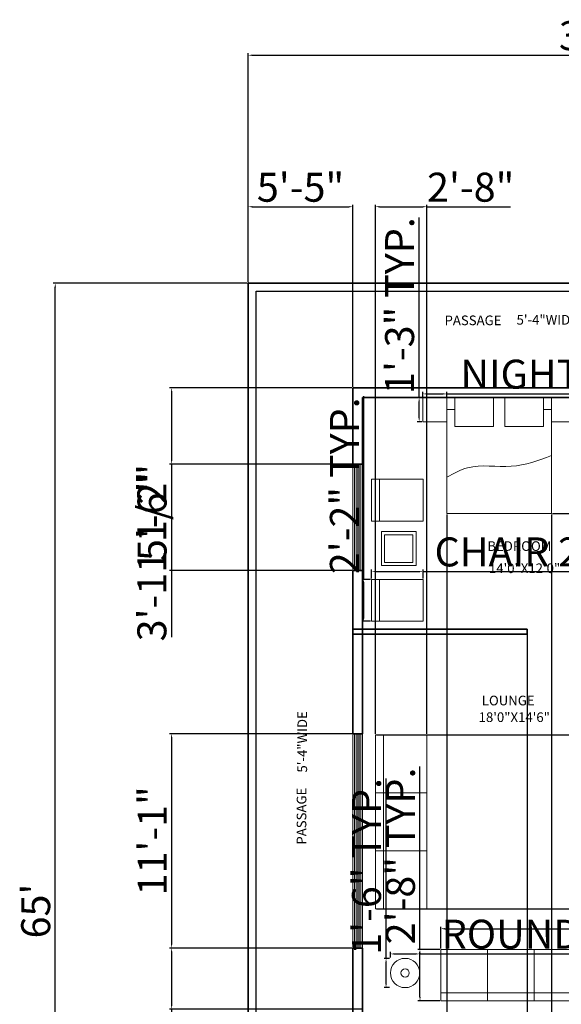
# Model space of a CAD drawing. Units: inches. Extents: x 2484 to 3244, y 1684 to 2692.
# Tile 2 of 3: x 2484 to 2821, y 2081 to 2692. Entities that reach past the tile are written whole.
import ezdxf

# ---------------------------------------------------------------- set-up
doc = ezdxf.new("R2010")
doc.units = ezdxf.units.IN
doc.layers.get('0').update_dxf_attribs({"color": 120})
for name, color, linetype, lineweight in [('A-ANNO-DIMS', 2, 'Continuous', 18), ('A-AREA-IDEN', 2, 'Continuous', 18), ('A-FURN', 40, 'Continuous', 18), ('A-GLAZ', 4, 'Continuous', 13), ('A-WALL', 120, 'Continuous', 35), ('C-PROP', 120, 'Continuous', 35), ('C-SITE', 120, 'Continuous', 25)]:
    doc.layers.add(name, color=color, linetype=linetype, lineweight=lineweight)
doc.styles.get("Standard").update_dxf_attribs({"font": 'arial.ttf'})
doc.dimstyles.new('ISO-25', dxfattribs={"dimtxt": 18, "dimasz": 2.5, "dimexe": 1.25, "dimexo": 0.625, "dimtad": 1, "dimdec": 0, "dimlunit": 3, "dimtxsty": 'Standard', "dimcen": 2.5, "dimadec": 0, "dimazin": 0, "dimtfac": 1, "dimtdec": 0, "dimtmove": 0, "dimatfit": 3, "dimfxl": 1, "dimarcsym": 0})

# ---------------------------------------------------------------- blocks, each defined once
blk = doc.blocks.new('*D1')
at = {"layer": 'A-ANNO-DIMS', "color": 0, "lineweight": -2, "transparency": 16777216}
for p, q in [((2626.09, 2529.34), (2626.09, 2671.64)), ((2628.59, 2670.39), (3043.59, 2670.39)), ((3046.09, 2529.34), (3046.09, 2671.64))]:
    blk.add_line(p, q, dxfattribs=at)
at = {"layer": 'A-ANNO-DIMS', "color": 0, "transparency": 16777216}
for points in [[(2628.59, 2670.81), (2628.59, 2669.97), (2626.09, 2670.39)], [(3043.59, 2670.81), (3043.59, 2669.97), (3046.09, 2670.39)]]:
    blk.add_solid(points, dxfattribs=at)
at = {"layer": 'Defpoints', "color": 0, "transparency": 16777216}
for p in [(3046.09, 2670.39), (2626.09, 2528.71), (3046.09, 2528.71)]:
    blk.add_point(p, dxfattribs=at)
at = {"layer": 'A-ANNO-DIMS', "color": 0, "transparency": 16777216, "insert": (2836.09, 2680.21), "char_height": 18, "attachment_point": 5}
blk.add_mtext("35'", dxfattribs=at)
blk = doc.blocks.new('*D2')
at = {"layer": 'A-ANNO-DIMS', "color": 0, "lineweight": -2, "transparency": 16777216}
for p, q in [((2625.46, 2528.71), (2505.02, 2528.71)), ((2506.27, 1751.21), (2506.27, 2526.21)), ((2625.46, 1748.71), (2505.02, 1748.71))]:
    blk.add_line(p, q, dxfattribs=at)
at = {"layer": 'A-ANNO-DIMS', "color": 0, "transparency": 16777216}
for points in [[(2505.85, 2526.21), (2506.68, 2526.21), (2506.27, 2528.71)], [(2505.85, 1751.21), (2506.68, 1751.21), (2506.27, 1748.71)]]:
    blk.add_solid(points, dxfattribs=at)
at = {"layer": 'Defpoints', "color": 0, "transparency": 16777216}
for p in [(2506.27, 2528.71), (2626.09, 2528.71), (2626.09, 1748.71)]:
    blk.add_point(p, dxfattribs=at)
at = {"layer": 'A-ANNO-DIMS', "color": 0, "transparency": 16777216, "insert": (2496.45, 2138.71), "char_height": 18, "attachment_point": 5, "rotation": 90}
blk.add_mtext("65'", dxfattribs=at)
blk = doc.blocks.new('SOFA-3')
for p, q in [((0.07, 0), (0.07, 32)), ((0.07, 32), (86.07, 32)), ((29.07, 0), (29.07, 32)), ((58.07, 0), (58.07, 32)), ((86.07, 32), (86.07, 0)), ((0.07, 0), (0, 5)), ((0, 5), (86.07, 5)), ((0.07, 0), (0.07, 5)), ((86.07, 0), (0.07, 0))]:
    blk.add_line(p, q)
blk = doc.blocks.new('CHAIR')
for p, q in [((0, 26), (5, 26)), ((5, 26), (5, 0))]:
    blk.add_line(p, q)
blk.add_lwpolyline([(0, 0), (32, 0), (32, 26), (0, 26)], close=True)
blk = doc.blocks.new('TABLE-ROUND')
for radius in [9.1, 2.6]:
    blk.add_circle((0, 0), radius)
blk = doc.blocks.new('NIGHTSTAND-15')
blk.add_lwpolyline([(15, 15), (0, 15), (0, 0), (15, 0)], close=True)
blk = doc.blocks.new('*D9')
at = {"layer": 'A-ANNO-DIMS', "color": 0, "lineweight": -2, "transparency": 16777216}
for p, q in [((2714.44, 2109.91), (2714.44, 2113.27)), ((2716.94, 2112.02), (2730.14, 2112.02)), ((2732.64, 2109.91), (2732.64, 2113.27)), ((2732.64, 2112.02), (3096.69, 2112.02))]:
    blk.add_line(p, q, dxfattribs=at)
at = {"layer": 'A-ANNO-DIMS', "color": 0, "transparency": 16777216}
for points in [[(2716.94, 2112.44), (2716.94, 2111.6), (2714.44, 2112.02)], [(2730.14, 2112.44), (2730.14, 2111.6), (2732.64, 2112.02)]]:
    blk.add_solid(points, dxfattribs=at)
at = {"layer": 'Defpoints', "color": 0, "transparency": 16777216}
for p in [(2732.64, 2112.02), (2714.44, 2109.29), (2732.64, 2109.29)]:
    blk.add_point(p, dxfattribs=at)
at = {"layer": 'A-ANNO-DIMS', "color": 0, "transparency": 16777216, "insert": (2915.92, 2121.96), "char_height": 18, "attachment_point": 5}
blk.add_mtext('ROUND SIDE TABLE 1\'-6" TYP.', dxfattribs=at)
blk = doc.blocks.new('*D10')
at = {"layer": 'A-ANNO-DIMS', "color": 0, "lineweight": -2, "transparency": 16777216}
for p, q in [((2711.71, 2109.29), (2711.71, 2221.06)), ((2713.81, 2109.29), (2710.46, 2109.29)), ((2711.71, 2093.58), (2711.71, 2106.79)), ((2713.81, 2091.08), (2710.46, 2091.08))]:
    blk.add_line(p, q, dxfattribs=at)
at = {"layer": 'A-ANNO-DIMS', "color": 0, "transparency": 16777216}
for points in [[(2711.29, 2106.79), (2712.12, 2106.79), (2711.71, 2109.29)], [(2711.29, 2093.58), (2712.12, 2093.58), (2711.71, 2091.08)]]:
    blk.add_solid(points, dxfattribs=at)
at = {"layer": 'Defpoints', "color": 0, "transparency": 16777216}
for p in [(2711.71, 2109.29), (2714.44, 2109.29), (2714.44, 2091.08)]:
    blk.add_point(p, dxfattribs=at)
at = {"layer": 'A-ANNO-DIMS', "color": 0, "transparency": 16777216, "insert": (2701.89, 2166.43), "char_height": 18, "attachment_point": 5, "rotation": 90}
blk.add_mtext('1\'-6" TYP.', dxfattribs=at)
blk = doc.blocks.new('*D13')
at = {"layer": 'A-ANNO-DIMS', "color": 0, "lineweight": -2, "transparency": 16777216}
for p, q in [((2745.68, 2115.42), (2745.68, 2128.95)), ((2831.75, 2115.42), (2831.75, 2128.95)), ((2748.18, 2127.7), (2829.25, 2127.7)), ((2831.75, 2127.7), (3115.68, 2127.7))]:
    blk.add_line(p, q, dxfattribs=at)
at = {"layer": 'A-ANNO-DIMS', "color": 0, "transparency": 16777216}
for points in [[(2748.18, 2128.12), (2748.18, 2127.28), (2745.68, 2127.7)], [(2829.25, 2128.12), (2829.25, 2127.28), (2831.75, 2127.7)]]:
    blk.add_solid(points, dxfattribs=at)
at = {"layer": 'Defpoints', "color": 0, "transparency": 16777216}
for p in [(2831.75, 2127.7), (2745.68, 2114.79), (2831.75, 2114.79)]:
    blk.add_point(p, dxfattribs=at)
at = {"layer": 'A-ANNO-DIMS', "color": 0, "transparency": 16777216, "insert": (2974.96, 2137.65), "char_height": 18, "attachment_point": 5}
blk.add_mtext('3-SEAT SOFA 7\'-2" TYP.', dxfattribs=at)
blk = doc.blocks.new('*D14')
at = {"layer": 'A-ANNO-DIMS', "color": 0, "lineweight": -2, "transparency": 16777216}
for p, q in [((2732.77, 2114.79), (2732.77, 2228.57)), ((2745.06, 2114.79), (2731.52, 2114.79)), ((2732.77, 2085.29), (2732.77, 2112.29)), ((2745.06, 2082.79), (2731.52, 2082.79))]:
    blk.add_line(p, q, dxfattribs=at)
at = {"layer": 'A-ANNO-DIMS', "color": 0, "transparency": 16777216}
for points in [[(2732.36, 2112.29), (2733.19, 2112.29), (2732.77, 2114.79)], [(2732.36, 2085.29), (2733.19, 2085.29), (2732.77, 2082.79)]]:
    blk.add_solid(points, dxfattribs=at)
at = {"layer": 'Defpoints', "color": 0, "transparency": 16777216}
for p in [(2732.77, 2114.79), (2745.68, 2114.79), (2745.68, 2082.79)]:
    blk.add_point(p, dxfattribs=at)
at = {"layer": 'A-ANNO-DIMS', "color": 0, "transparency": 16777216, "insert": (2722.96, 2172.93), "char_height": 18, "attachment_point": 5, "rotation": 90}
blk.add_mtext('2\'-8" TYP.', dxfattribs=at)
blk = doc.blocks.new('*D17')
at = {"layer": 'A-ANNO-DIMS', "color": 0, "lineweight": -2, "transparency": 16777216}
for p, q in [((2702.65, 2345.36), (2702.65, 2350.79)), ((2705.15, 2349.54), (2732.15, 2349.54)), ((2734.65, 2345.36), (2734.65, 2350.79)), ((2734.65, 2349.54), (2933.13, 2349.54))]:
    blk.add_line(p, q, dxfattribs=at)
at = {"layer": 'A-ANNO-DIMS', "color": 0, "transparency": 16777216}
for points in [[(2705.15, 2349.96), (2705.15, 2349.12), (2702.65, 2349.54)], [(2732.15, 2349.96), (2732.15, 2349.12), (2734.65, 2349.54)]]:
    blk.add_solid(points, dxfattribs=at)
at = {"layer": 'Defpoints', "color": 0, "transparency": 16777216}
for p in [(2734.65, 2349.54), (2702.65, 2344.74), (2734.65, 2344.74)]:
    blk.add_point(p, dxfattribs=at)
at = {"layer": 'A-ANNO-DIMS', "color": 0, "transparency": 16777216, "insert": (2835.14, 2359.47), "char_height": 18, "attachment_point": 5}
blk.add_mtext('CHAIR 2\'-8" TYP.', dxfattribs=at)
blk = doc.blocks.new('*D18')
at = {"layer": 'A-ANNO-DIMS', "color": 0, "lineweight": -2, "transparency": 16777216}
for p, q in [((2697.85, 2344.74), (2697.85, 2458.51)), ((2702.02, 2344.74), (2696.6, 2344.74)), ((2697.85, 2321.24), (2697.85, 2342.24)), ((2702.02, 2318.74), (2696.6, 2318.74))]:
    blk.add_line(p, q, dxfattribs=at)
at = {"layer": 'A-ANNO-DIMS', "color": 0, "transparency": 16777216}
for points in [[(2697.43, 2342.24), (2698.26, 2342.24), (2697.85, 2344.74)], [(2697.43, 2321.24), (2698.26, 2321.24), (2697.85, 2318.74)]]:
    blk.add_solid(points, dxfattribs=at)
at = {"layer": 'Defpoints', "color": 0, "transparency": 16777216}
for p in [(2697.85, 2344.74), (2702.65, 2344.74), (2702.65, 2318.74)]:
    blk.add_point(p, dxfattribs=at)
at = {"layer": 'A-ANNO-DIMS', "color": 0, "transparency": 16777216, "insert": (2688.18, 2402.88), "char_height": 18, "attachment_point": 5, "rotation": 90}
blk.add_mtext('2\'-2" TYP.', dxfattribs=at)
blk = doc.blocks.new('*D19')
at = {"layer": 'A-ANNO-DIMS', "color": 0, "lineweight": -2, "transparency": 16777216}
for p, q in [((2734.51, 2458.34), (2734.51, 2461.21)), ((2737.01, 2459.96), (2747.01, 2459.96)), ((2749.51, 2458.34), (2749.51, 2461.21)), ((2749.51, 2459.96), (3032.54, 2459.96))]:
    blk.add_line(p, q, dxfattribs=at)
at = {"layer": 'A-ANNO-DIMS', "color": 0, "transparency": 16777216}
for points in [[(2737.01, 2460.38), (2737.01, 2459.55), (2734.51, 2459.96)], [(2747.01, 2460.38), (2747.01, 2459.55), (2749.51, 2459.96)]]:
    blk.add_solid(points, dxfattribs=at)
at = {"layer": 'Defpoints', "color": 0, "transparency": 16777216}
for p in [(2749.51, 2459.96), (2734.51, 2457.71), (2749.51, 2457.71)]:
    blk.add_point(p, dxfattribs=at)
at = {"layer": 'A-ANNO-DIMS', "color": 0, "transparency": 16777216, "insert": (2892.27, 2469.9), "char_height": 18, "attachment_point": 5}
blk.add_mtext('NIGHTSTAND 1\'-3" TYP.', dxfattribs=at)
blk = doc.blocks.new('*D20')
at = {"layer": 'A-ANNO-DIMS', "color": 0, "lineweight": -2, "transparency": 16777216}
for p, q in [((2732.26, 2457.71), (2732.26, 2569.49)), ((2733.88, 2457.71), (2731.01, 2457.71)), ((2732.26, 2445.21), (2732.26, 2455.21)), ((2733.88, 2442.71), (2731.01, 2442.71))]:
    blk.add_line(p, q, dxfattribs=at)
at = {"layer": 'A-ANNO-DIMS', "color": 0, "transparency": 16777216}
for points in [[(2731.84, 2455.21), (2732.67, 2455.21), (2732.26, 2457.71)], [(2731.84, 2445.21), (2732.67, 2445.21), (2732.26, 2442.71)]]:
    blk.add_solid(points, dxfattribs=at)
at = {"layer": 'Defpoints', "color": 0, "transparency": 16777216}
for p in [(2732.26, 2457.71), (2734.51, 2457.71), (2734.51, 2442.71)]:
    blk.add_point(p, dxfattribs=at)
at = {"layer": 'A-ANNO-DIMS', "color": 0, "transparency": 16777216, "insert": (2722.44, 2514.85), "char_height": 18, "attachment_point": 5, "rotation": 90}
blk.add_mtext('1\'-3" TYP.', dxfattribs=at)
blk = doc.blocks.new('*D21')
at = {"layer": 'A-ANNO-DIMS', "color": 0, "lineweight": -2, "transparency": 16777216}
for p, q in [((2749.51, 2385.09), (2749.51, 1699.91)), ((2814.51, 2385.09), (2814.51, 1699.91)), ((2752.01, 1701.16), (2812.01, 1701.16))]:
    blk.add_line(p, q, dxfattribs=at)
at = {"layer": 'A-ANNO-DIMS', "color": 0, "transparency": 16777216}
for points in [[(2752.01, 1701.58), (2752.01, 1700.75), (2749.51, 1701.16)], [(2812.01, 1701.58), (2812.01, 1700.75), (2814.51, 1701.16)]]:
    blk.add_solid(points, dxfattribs=at)
at = {"layer": 'Defpoints', "color": 0, "transparency": 16777216}
for p in [(2749.51, 2385.71), (2814.51, 2385.71), (2814.51, 1701.16)]:
    blk.add_point(p, dxfattribs=at)
at = {"layer": 'A-ANNO-DIMS', "color": 0, "transparency": 16777216, "insert": (2782.01, 1710.94), "char_height": 18, "attachment_point": 5}
blk.add_mtext('5\'-5"', dxfattribs=at)
blk = doc.blocks.new('*D22')
at = {"layer": 'A-ANNO-DIMS', "color": 0, "lineweight": -2, "transparency": 16777216}
for p, q in [((2815.13, 2457.71), (3094.89, 2457.71)), ((3093.64, 2388.21), (3093.64, 2455.21)), ((2815.13, 2385.71), (3094.89, 2385.71))]:
    blk.add_line(p, q, dxfattribs=at)
at = {"layer": 'A-ANNO-DIMS', "color": 0, "transparency": 16777216}
for points in [[(3093.22, 2455.21), (3094.05, 2455.21), (3093.64, 2457.71)], [(3093.22, 2388.21), (3094.05, 2388.21), (3093.64, 2385.71)]]:
    blk.add_solid(points, dxfattribs=at)
at = {"layer": 'Defpoints', "color": 0, "transparency": 16777216}
for p in [(2814.51, 2457.71), (3093.64, 2457.71), (2814.51, 2385.71)]:
    blk.add_point(p, dxfattribs=at)
at = {"layer": 'A-ANNO-DIMS', "color": 0, "transparency": 16777216, "insert": (3083.82, 2421.71), "char_height": 18, "attachment_point": 5, "rotation": 90}
blk.add_mtext('6\'-0"', dxfattribs=at)
blk = doc.blocks.new('*D25')
at = {"layer": 'A-ANNO-DIMS', "color": 0, "lineweight": -2, "transparency": 16777216}
for p, q in [((2690.46, 2416.35), (2577.29, 2416.35)), ((2578.54, 2413.85), (2578.54, 2352.67)), ((2690.46, 2350.17), (2577.29, 2350.17))]:
    blk.add_line(p, q, dxfattribs=at)
at = {"layer": 'A-ANNO-DIMS', "color": 0, "transparency": 16777216}
for points in [[(2578.12, 2413.85), (2578.95, 2413.85), (2578.54, 2416.35)], [(2578.12, 2352.67), (2578.95, 2352.67), (2578.54, 2350.17)]]:
    blk.add_solid(points, dxfattribs=at)
at = {"layer": 'Defpoints', "color": 0, "transparency": 16777216}
for p in [(2691.09, 2416.35), (2578.54, 2350.17), (2691.09, 2350.17)]:
    blk.add_point(p, dxfattribs=at)
at = {"layer": 'A-ANNO-DIMS', "color": 0, "transparency": 16777216, "insert": (2568.72, 2383.26), "char_height": 18, "attachment_point": 5, "rotation": 90}
blk.add_mtext('5\'-6"', dxfattribs=at)
blk = doc.blocks.new('*D26')
at = {"layer": 'A-ANNO-DIMS', "color": 0, "lineweight": -2, "transparency": 16777216}
for p, q in [((2690.46, 2248.87), (2577.29, 2248.87)), ((2578.54, 2246.37), (2578.54, 2118.2)), ((2690.46, 2115.7), (2577.29, 2115.7))]:
    blk.add_line(p, q, dxfattribs=at)
at = {"layer": 'A-ANNO-DIMS', "color": 0, "transparency": 16777216}
for points in [[(2578.12, 2246.37), (2578.95, 2246.37), (2578.54, 2248.87)], [(2578.12, 2118.2), (2578.95, 2118.2), (2578.54, 2115.7)]]:
    blk.add_solid(points, dxfattribs=at)
at = {"layer": 'Defpoints', "color": 0, "transparency": 16777216}
for p in [(2691.09, 2248.87), (2578.54, 2115.7), (2691.09, 2115.7)]:
    blk.add_point(p, dxfattribs=at)
at = {"layer": 'A-ANNO-DIMS', "color": 0, "transparency": 16777216, "insert": (2568.88, 2182.29), "char_height": 18, "attachment_point": 5, "rotation": 90}
blk.add_mtext('11\'-1"', dxfattribs=at)
blk = doc.blocks.new('*D27')
at = {"layer": 'A-ANNO-DIMS', "color": 0, "lineweight": -2, "transparency": 16777216}
for p, q in [((2690.46, 2463.71), (2577.29, 2463.71)), ((2578.54, 2461.21), (2578.54, 2418.85)), ((2690.46, 2416.35), (2577.29, 2416.35)), ((2578.54, 2416.35), (2578.54, 2308.84))]:
    blk.add_line(p, q, dxfattribs=at)
at = {"layer": 'A-ANNO-DIMS', "color": 0, "transparency": 16777216}
for points in [[(2578.12, 2461.21), (2578.95, 2461.21), (2578.54, 2463.71)], [(2578.12, 2418.85), (2578.95, 2418.85), (2578.54, 2416.35)]]:
    blk.add_solid(points, dxfattribs=at)
at = {"layer": 'Defpoints', "color": 0, "transparency": 16777216}
for p in [(2691.09, 2463.71), (2578.54, 2416.35), (2691.09, 2416.35)]:
    blk.add_point(p, dxfattribs=at)
at = {"layer": 'A-ANNO-DIMS', "color": 0, "transparency": 16777216, "insert": (2568.6, 2361.35), "char_height": 18, "attachment_point": 5, "rotation": 90}
blk.add_mtext('3\'-11 1/2"', dxfattribs=at)
blk = doc.blocks.new('*D28')
at = {"layer": 'A-ANNO-DIMS', "color": 0, "lineweight": -2, "transparency": 16777216}
for p, q in [((2690.46, 2115.7), (2577.29, 2115.7)), ((2578.54, 2113.2), (2578.54, 2080.21)), ((2696.46, 2077.71), (2577.29, 2077.71)), ((2578.54, 2077.71), (2578.54, 2026.13))]:
    blk.add_line(p, q, dxfattribs=at)
at = {"layer": 'A-ANNO-DIMS', "color": 0, "transparency": 16777216}
for points in [[(2578.12, 2113.2), (2578.95, 2113.2), (2578.54, 2115.7)], [(2578.12, 2080.21), (2578.95, 2080.21), (2578.54, 2077.71)]]:
    blk.add_solid(points, dxfattribs=at)
at = {"layer": 'Defpoints', "color": 0, "transparency": 16777216}
for p in [(2691.09, 2115.7), (2578.54, 2077.71), (2697.09, 2077.71)]:
    blk.add_point(p, dxfattribs=at)
at = {"layer": 'A-ANNO-DIMS', "color": 0, "transparency": 16777216, "insert": (2568.72, 2050.67), "char_height": 18, "attachment_point": 5, "rotation": 90}
blk.add_mtext('3\'-2"', dxfattribs=at)
blk = doc.blocks.new('*D31')
at = {"layer": 'A-ANNO-DIMS', "color": 0, "lineweight": -2, "transparency": 16777216}
for p, q in [((2705.68, 2248.09), (3094.89, 2248.09)), ((3093.64, 2245.59), (3093.64, 2142.59)), ((2705.68, 2140.09), (3094.89, 2140.09))]:
    blk.add_line(p, q, dxfattribs=at)
at = {"layer": 'A-ANNO-DIMS', "color": 0, "transparency": 16777216}
for points in [[(3093.22, 2245.59), (3094.05, 2245.59), (3093.64, 2248.09)], [(3093.22, 2142.59), (3094.05, 2142.59), (3093.64, 2140.09)]]:
    blk.add_solid(points, dxfattribs=at)
at = {"layer": 'Defpoints', "color": 0, "transparency": 16777216}
for p in [(2705.05, 2248.09), (2705.05, 2140.09), (3093.64, 2140.09)]:
    blk.add_point(p, dxfattribs=at)
at = {"layer": 'A-ANNO-DIMS', "color": 0, "transparency": 16777216, "insert": (3083.82, 2194.09), "char_height": 18, "attachment_point": 5, "rotation": 90}
blk.add_mtext('9\'-0"', dxfattribs=at)
blk = doc.blocks.new('*D32')
at = {"layer": 'A-ANNO-DIMS', "color": 0, "lineweight": -2, "transparency": 16777216}
for p, q in [((2705.05, 2248.72), (2705.05, 2577.51)), ((2707.55, 2576.26), (2734.55, 2576.26)), ((2737.05, 2248.72), (2737.05, 2577.51)), ((2737.05, 2576.26), (2788.96, 2576.26))]:
    blk.add_line(p, q, dxfattribs=at)
at = {"layer": 'A-ANNO-DIMS', "color": 0, "transparency": 16777216}
for points in [[(2707.55, 2576.68), (2707.55, 2575.85), (2705.05, 2576.26)], [(2734.55, 2576.68), (2734.55, 2575.85), (2737.05, 2576.26)]]:
    blk.add_solid(points, dxfattribs=at)
at = {"layer": 'Defpoints', "color": 0, "transparency": 16777216}
for p in [(2737.05, 2576.26), (2705.05, 2248.09), (2737.05, 2248.09)]:
    blk.add_point(p, dxfattribs=at)
at = {"layer": 'A-ANNO-DIMS', "color": 0, "transparency": 16777216, "insert": (2764.26, 2586.08), "char_height": 18, "attachment_point": 5}
blk.add_mtext('2\'-8"', dxfattribs=at)
blk = doc.blocks.new('*D35')
at = {"layer": 'A-ANNO-DIMS', "color": 0, "lineweight": -2, "transparency": 16777216}
for p, q in [((2626.09, 2529.34), (2626.09, 2577.51)), ((2628.59, 2576.26), (2688.59, 2576.26)), ((2691.09, 2464.34), (2691.09, 2577.51))]:
    blk.add_line(p, q, dxfattribs=at)
at = {"layer": 'A-ANNO-DIMS', "color": 0, "transparency": 16777216}
for points in [[(2628.59, 2576.68), (2628.59, 2575.85), (2626.09, 2576.26)], [(2688.59, 2576.68), (2688.59, 2575.85), (2691.09, 2576.26)]]:
    blk.add_solid(points, dxfattribs=at)
at = {"layer": 'Defpoints', "color": 0, "transparency": 16777216}
for p in [(2691.09, 2576.26), (2626.09, 2528.71), (2691.09, 2463.71)]:
    blk.add_point(p, dxfattribs=at)
at = {"layer": 'A-ANNO-DIMS', "color": 0, "transparency": 16777216, "insert": (2658.59, 2586.04), "char_height": 18, "attachment_point": 5}
blk.add_mtext('5\'-5"', dxfattribs=at)
blk = doc.blocks.new('*D37')
at = {"layer": 'A-ANNO-DIMS', "color": 0, "lineweight": -2, "transparency": 16777216}
for p, q in [((2799.42, 2313.09), (2799.42, 1699.91)), ((2851.28, 2313.09), (2851.28, 1699.91)), ((2801.92, 1701.16), (2848.78, 1701.16))]:
    blk.add_line(p, q, dxfattribs=at)
at = {"layer": 'A-ANNO-DIMS', "color": 0, "transparency": 16777216}
for points in [[(2801.92, 1701.58), (2801.92, 1700.75), (2799.42, 1701.16)], [(2848.78, 1701.58), (2848.78, 1700.75), (2851.28, 1701.16)]]:
    blk.add_solid(points, dxfattribs=at)
at = {"layer": 'Defpoints', "color": 0, "transparency": 16777216}
for p in [(2799.42, 2313.71), (2851.28, 2313.71), (2851.28, 1701.16)]:
    blk.add_point(p, dxfattribs=at)
at = {"layer": 'A-ANNO-DIMS', "color": 0, "transparency": 16777216, "insert": (2825.35, 1710.79), "char_height": 18, "attachment_point": 5}
blk.add_mtext('4\'-4"', dxfattribs=at)

msp = doc.modelspace()

# ---------------------------------------------------------------- linework, layer by layer
at = {"layer": 'A-FURN'}
for p, q in [((2749.51, 2450.21), (2754.51, 2450.21)), ((2814.51, 2450.21), (2809.51, 2450.21)), ((2705.05, 2248.09), (2737.05, 2248.09)), ((2705.05, 2140.09), (2705.05, 2248.09)), ((2705.05, 2248.09), (2710.05, 2248.09)), ((2710.05, 2248.09), (2710.05, 2140.09)), ((2737.05, 2248.09), (2737.05, 2140.09)), ((2705.05, 2212.09), (2737.05, 2212.09)), ((2705.05, 2176.09), (2737.05, 2176.09)), ((2737.05, 2140.09), (2705.05, 2140.09))]:
    msp.add_line(p, q, dxfattribs=at)
for points in [[(2814.51, 2457.71), (2749.51, 2457.71), (2749.51, 2385.71), (2814.51, 2385.71)], [(2754.51, 2457.71), (2778.51, 2457.71), (2778.51, 2439.71), (2754.51, 2439.71)], [(2785.51, 2457.71), (2809.51, 2457.71), (2809.51, 2439.71), (2785.51, 2439.71)], [(2708.79, 2374.47), (2730.33, 2374.47), (2730.33, 2353.32), (2708.79, 2353.32)], [(2710.79, 2372.47), (2728.33, 2372.47), (2728.33, 2355.32), (2710.79, 2355.32)]]:
    msp.add_lwpolyline(points, close=True, dxfattribs=at)
msp.add_open_spline([(2749.51, 2408.2), (2753.7, 2410.56), (2765.96, 2417.43), (2789.54, 2412.39), (2806.32, 2418.65), (2814.51, 2421.71)], degree=3, knots=[0, 0, 0, 0, 14.134483, 41.285729, 67.192601, 67.192601, 67.192601, 67.192601], dxfattribs=at)
at = {"layer": 'A-GLAZ'}
for p, q in [((2691.09, 2416.35), (2691.09, 2350.17)), ((2692.09, 2416.35), (2692.09, 2350.17)), ((2693.09, 2416.35), (2693.09, 2350.17)), ((2694.09, 2416.35), (2694.09, 2350.17)), ((2695.09, 2416.35), (2695.09, 2350.17)), ((2696.09, 2416.35), (2696.09, 2350.17)), ((2697.09, 2416.35), (2697.09, 2350.17)), ((2691.09, 2248.87), (2691.09, 2115.7)), ((2692.09, 2248.87), (2692.09, 2115.7)), ((2693.09, 2248.87), (2693.09, 2115.7)), ((2694.09, 2248.87), (2694.09, 2115.7)), ((2695.09, 2248.87), (2695.09, 2115.7)), ((2696.09, 2248.87), (2696.09, 2115.7)), ((2697.09, 2248.87), (2697.09, 2115.7))]:
    msp.add_line(p, q, dxfattribs=at)
at = {"layer": 'A-WALL'}
for p, q in [((2691.09, 2463.71), (2896.09, 2463.71)), ((2691.09, 2416.35), (2691.09, 2463.71)), ((2697.09, 2457.71), (2893.09, 2457.71)), ((2697.09, 2416.35), (2697.09, 2457.71)), ((2691.09, 2416.35), (2697.09, 2416.35)), ((2691.09, 2350.17), (2697.09, 2350.17)), ((2691.09, 2248.87), (2691.09, 2350.17)), ((2697.09, 2248.87), (2697.09, 2350.17)), ((2691.09, 2313.71), (2799.42, 2313.71)), ((2799.42, 2313.71), (2799.42, 2310.71)), ((2691.09, 2310.71), (2799.42, 2310.71)), ((2691.09, 2248.87), (2697.09, 2248.87)), ((2691.09, 1970.71), (2691.09, 2115.7)), ((2691.09, 2115.7), (2697.09, 2115.7)), ((2697.09, 1979.71), (2697.09, 2115.7))]:
    msp.add_line(p, q, dxfattribs=at)
at = {"layer": 'C-PROP'}
msp.add_lwpolyline([(2626.09, 2528.71), (3046.09, 2528.71), (3046.09, 1748.71), (2626.09, 1748.71)], close=True, dxfattribs=at)
at = {"layer": 'C-SITE'}
for p, q in [((2631.09, 2523.71), (3041.09, 2523.71)), ((2631.09, 1753.71), (2631.09, 2523.71))]:
    msp.add_line(p, q, dxfattribs=at)

# ---------------------------------------------------------------- block references
at = {"layer": 'A-FURN'}
for name, p in [('NIGHTSTAND-15', (2734.51, 2442.71)), ('NIGHTSTAND-15', (2814.51, 2442.71)), ('CHAIR', (2702.65, 2380.92)), ('CHAIR', (2702.65, 2318.74)), ('SOFA-3', (2745.68, 2082.79)), ('TABLE-ROUND', (2723.54, 2100.19))]:
    msp.add_blockref(name, p, dxfattribs=at)

# ---------------------------------------------------------------- texts
at = {"layer": 'A-AREA-IDEN'}
for tag, p in [('PASSAGE', (2748.02, 2502.68)), ('5\'-4"WIDE', (2792.76, 2503.01)), ('BEDROOM', (2774.61, 2362.42)), ('14\'0"X12\'0"', (2775.6, 2348.64)), ('LOUNGE', (2771.17, 2266.46)), ('18\'0"X14\'6"', (2769.2, 2256.12))]:
    msp.add_attdef(tag, p, '', height=6, dxfattribs=at)
for tag, p in [('5\'-4"WIDE', (2662.67, 2224.71)), ('PASSAGE', (2662.21, 2179.95))]:
    msp.add_attdef(tag, p, '', height=6, rotation=90, dxfattribs=at)

# ---------------------------------------------------------------- dimensions: what is measured, and where the dimension line sits
at = {"layer": 'A-ANNO-DIMS'}
for base, p1, p2, override, picture, middle in [((3046.09, 2670.39), (2626.09, 2528.71), (3046.09, 2528.71), {"dimclrd": 0, "dimclre": 0, "dimclrt": 0}, '*D1', (2836.09, 2680.21)), ((2691.09, 2576.26), (2626.09, 2528.71), (2691.09, 2463.71), {"dimdec": 1, "dimlfac": 1, "dimrnd": 0, "dimzin": 1, "dimdsep": 46, "dimlunit": 4, "dimfrac": 2}, '*D35', (2658.59, 2586.04)), ((2737.05, 2576.26), (2705.05, 2248.09), (2737.05, 2248.09), {"dimdec": 1, "dimlfac": 1, "dimrnd": 0, "dimzin": 1, "dimdsep": 46, "dimlunit": 4, "dimfrac": 2}, '*D32', (2764.26, 2586.08)), ((2814.51, 1701.16), (2749.51, 2385.71), (2814.51, 2385.71), {"dimdec": 1, "dimlfac": 1, "dimrnd": 0, "dimzin": 1, "dimdsep": 46, "dimlunit": 4, "dimfrac": 2}, '*D21', (2782.01, 1710.94)), ((2851.28, 1701.16), (2799.42, 2313.71), (2851.28, 2313.71), {"dimdec": 1, "dimlfac": 1, "dimrnd": 0, "dimzin": 1, "dimdsep": 46, "dimlunit": 4, "dimfrac": 2}, '*D37', (2825.35, 1710.79))]:
    dim = msp.add_linear_dim(base=base, p1=p1, p2=p2, dimstyle='ISO-25', override=override, dxfattribs=at)
    dim.commit()
    dim.dimension.update_dxf_attribs({"geometry": picture, "text_midpoint": middle})
for base, p1, p2, picture, middle in [((2732.26, 2457.71), (2734.51, 2442.71), (2734.51, 2457.71), '*D20', (2722.44, 2514.85)), ((2697.85, 2344.74), (2702.65, 2318.74), (2702.65, 2344.74), '*D18', (2688.18, 2402.88)), ((2732.77, 2114.79), (2745.68, 2082.79), (2745.68, 2114.79), '*D14', (2722.96, 2172.93)), ((2711.71, 2109.29), (2714.44, 2091.08), (2714.44, 2109.29), '*D10', (2701.89, 2166.43))]:
    dim = msp.add_linear_dim(base=base, p1=p1, p2=p2, angle=90, text='<> TYP.', dimstyle='ISO-25', override={"dimdec": 1, "dimlfac": 1, "dimrnd": 0, "dimzin": 1, "dimdsep": 46, "dimlunit": 4, "dimfrac": 2}, dxfattribs=at)
    dim.commit()
    dim.dimension.update_dxf_attribs({"geometry": picture, "text_midpoint": middle})
for base, p1, p2, override, picture, middle in [((2506.27, 2528.71), (2626.09, 1748.71), (2626.09, 2528.71), {"dimclrd": 0, "dimclre": 0, "dimclrt": 0}, '*D2', (2496.45, 2138.71)), ((2578.54, 2416.35), (2691.09, 2463.71), (2691.09, 2416.35), {"dimdec": 1, "dimlfac": 1, "dimrnd": 0, "dimzin": 1, "dimdsep": 46, "dimlunit": 4, "dimfrac": 2}, '*D27', (2568.6, 2361.35)), ((3093.64, 2457.71), (2814.51, 2385.71), (2814.51, 2457.71), {"dimdec": 1, "dimlfac": 1, "dimrnd": 0, "dimzin": 1, "dimdsep": 46, "dimlunit": 4, "dimfrac": 2}, '*D22', (3083.82, 2421.71)), ((2578.54, 2350.17), (2691.09, 2416.35), (2691.09, 2350.17), {"dimdec": 1, "dimlfac": 1, "dimrnd": 0, "dimzin": 1, "dimdsep": 46, "dimlunit": 4, "dimfrac": 2}, '*D25', (2568.72, 2383.26)), ((2578.54, 2115.7), (2691.09, 2248.87), (2691.09, 2115.7), {"dimdec": 1, "dimlfac": 1, "dimrnd": 0, "dimzin": 1, "dimdsep": 46, "dimlunit": 4, "dimfrac": 2}, '*D26', (2568.88, 2182.29)), ((3093.64, 2140.09), (2705.05, 2248.09), (2705.05, 2140.09), {"dimdec": 1, "dimlfac": 1, "dimrnd": 0, "dimzin": 1, "dimdsep": 46, "dimlunit": 4, "dimfrac": 2}, '*D31', (3083.82, 2194.09)), ((2578.54, 2077.71), (2691.09, 2115.7), (2697.09, 2077.71), {"dimdec": 1, "dimlfac": 1, "dimrnd": 0, "dimzin": 1, "dimdsep": 46, "dimlunit": 4, "dimfrac": 2}, '*D28', (2568.72, 2050.67))]:
    dim = msp.add_linear_dim(base=base, p1=p1, p2=p2, angle=90, dimstyle='ISO-25', override=override, dxfattribs=at)
    dim.commit()
    dim.dimension.update_dxf_attribs({"geometry": picture, "text_midpoint": middle})
for base, p1, p2, text, picture, middle in [((2749.51, 2459.96), (2734.51, 2457.71), (2749.51, 2457.71), 'NIGHTSTAND <> TYP.', '*D19', (2892.27, 2469.9)), ((2734.65, 2349.54), (2702.65, 2344.74), (2734.65, 2344.74), 'CHAIR <> TYP.', '*D17', (2835.14, 2359.47)), ((2732.64, 2112.02), (2714.44, 2109.29), (2732.64, 2109.29), 'ROUND SIDE TABLE <> TYP.', '*D9', (2915.92, 2121.96)), ((2831.75, 2127.7), (2745.68, 2114.79), (2831.75, 2114.79), '3-SEAT SOFA <> TYP.', '*D13', (2974.96, 2137.65))]:
    dim = msp.add_linear_dim(base=base, p1=p1, p2=p2, text=text, dimstyle='ISO-25', override={"dimdec": 1, "dimlfac": 1, "dimrnd": 0, "dimzin": 1, "dimdsep": 46, "dimlunit": 4, "dimfrac": 2}, dxfattribs=at)
    dim.commit()
    dim.dimension.update_dxf_attribs({"geometry": picture, "text_midpoint": middle})

doc.saveas('drawing.dxf')
